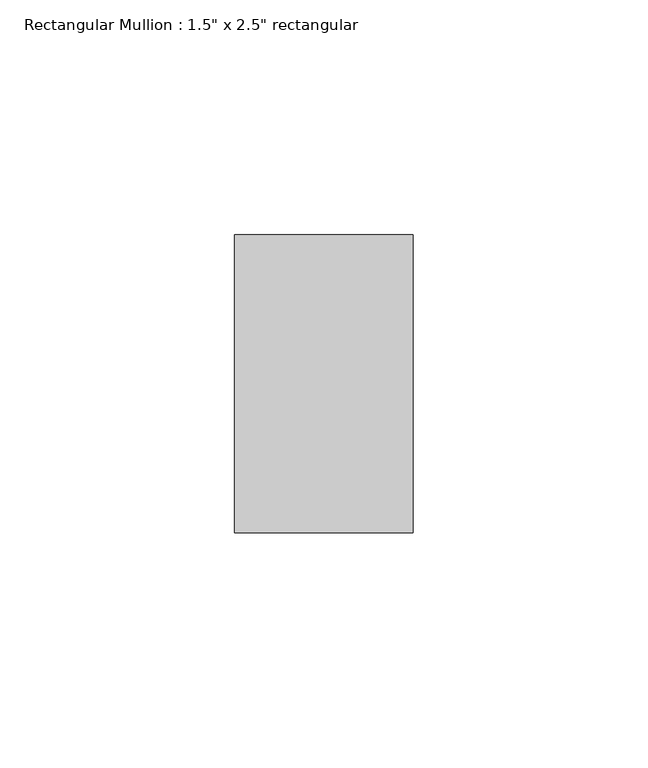
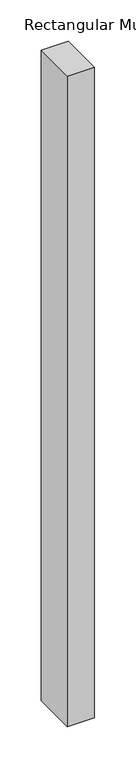
"""IFC4 building model written with IfcOpenShell, lengths in millimetres: member geometry."""

from ifc_helpers import new_model, si_unit, frame, origin, place, context, project, spatial, polyline, outline, extrude, source, transform, mapped, element, save


def member_32999801(model_context):
    return source(origin(), model_context, "Body", "SweptSolid", [
        extrude(outline(polyline([(0.0, 31.75), (0.0, -31.75), (-38.1, -31.75), (-38.1, 31.75), (0.0, 31.75)])), frame((0.0, 0.0, -965.2), z_axis=(0.0, 0.0, 1.0), x_axis=(1.0, 0.0, 0.0)), (0.0, 0.0, 1.0), 965.2),
    ])


if __name__ == "__main__":
    model = new_model("IFC4")
    model_context = context("Model", 3, world=origin())
    ifc_project = project(units=[si_unit("LENGTHUNIT", "METRE", prefix="MILLI")], contexts=[model_context])
    site = spatial("IfcSite", under=ifc_project)
    building = spatial("IfcBuilding", under=site)
    placement = place(None, origin())
    member_shape = member_32999801(model_context)
    element("IfcMember", 1, ObjectType="Rectangular Mullion : 1.5\" x 2.5\" rectangular", at=placement, inside=building, context=model_context, shape_type="MappedRepresentation", body=[
        mapped(member_shape, transform((0.0, 0.0, 0.0), x_axis=(1.0, 0.0, 0.0), y_axis=(0.0, 1.0, 0.0), z_axis=(0.0, 0.0, 1.0))),
    ])
    save(model, "model.ifc")

# Revit data of these elements
# Type "Rectangular Mullion : 1.5\" x 2.5\" rectangular"
#   built-in parameter 1007304 = 0.208333 (stored number, unit not read)
#   built-in parameter 1007301 = 0.0625 (stored number, unit not read)
#   built-in parameter 1007300 = 0.0625 (stored number, unit not read)
# Element 1 (IfcMember, "Rectangular Mullion : 1.5\" x 2.5\" rectangular")
#   Materials on its faces: "Aluminum"
# Materials
#   "Aluminum": class "Metal", colour RGB 247 247 247, transparency 0, Description = "Aluminum 6061", Cost = 0
